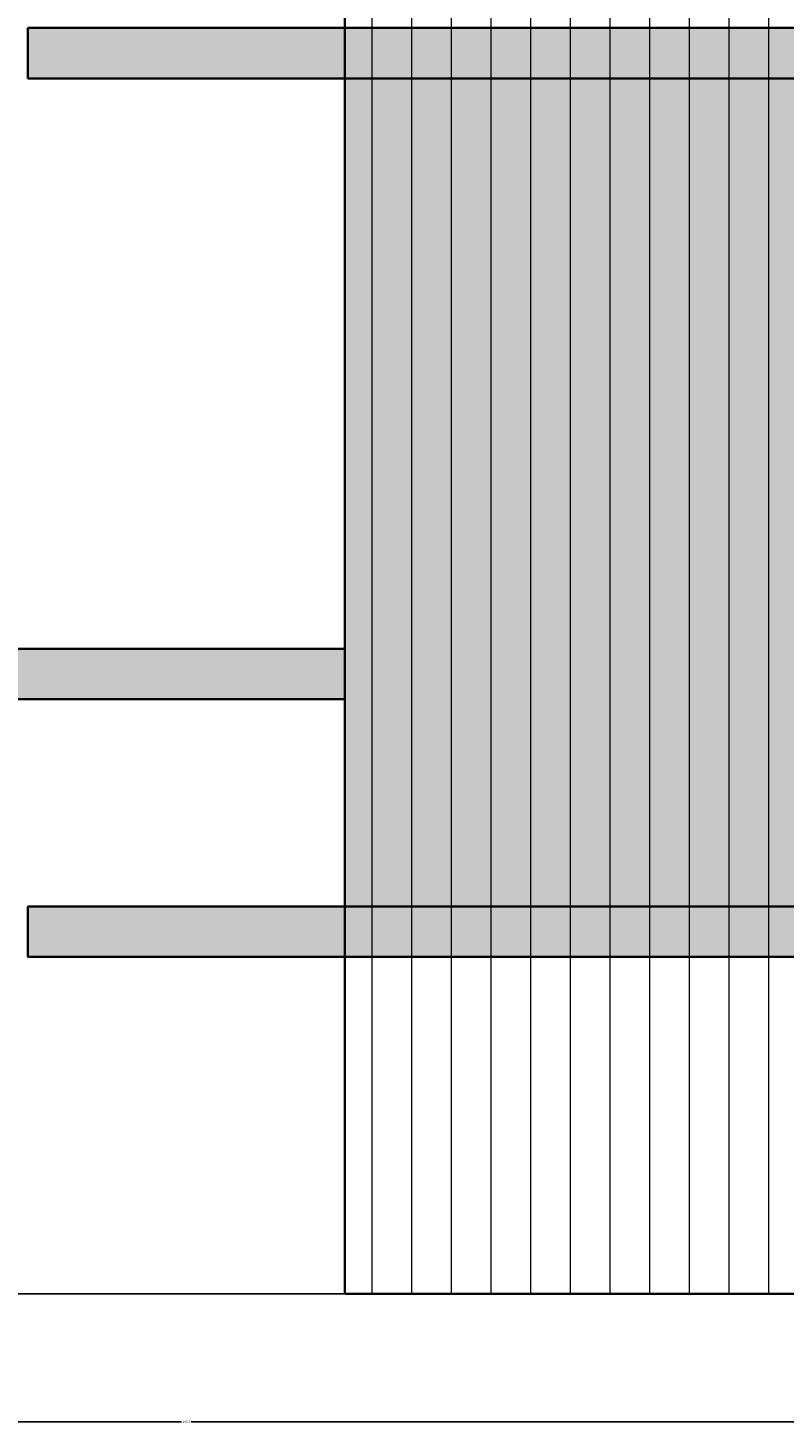
# Model space of a CAD drawing. Units: millimetres. Extents: x 446512 to 447461, y 70395 to 70610.
# Tile 33 of 39: x 447340 to 447401, y 70395 to 70507. Entities that reach past the tile are written whole.
import ezdxf

# ---------------------------------------------------------------- set-up
doc = ezdxf.new("R2010")
doc.units = ezdxf.units.MM
for name, color, linetype, lineweight in [('A-ANNO-DIMS', 2, 'Continuous', 18), ('A-FURN', 7, 'Continuous', 35), ('A-FURN-PATT', 38, 'Continuous', 13)]:
    doc.layers.add(name, color=color, linetype=linetype, lineweight=lineweight)
doc.styles.get("Standard").update_dxf_attribs({"font": 'arial.ttf'})
doc.dimstyles.get("Standard").update_dxf_attribs({"dimtxt": 0.18, "dimasz": 0.18, "dimexe": 0.18, "dimexo": 0.0625, "dimgap": 0.09, "dimtad": 0, "dimtih": 1, "dimtoh": 1, "dimdec": 4, "dimzin": 0, "dimdsep": 46, "dimtxsty": 'Standard', "dimcen": 0.09, "dimadec": 0, "dimazin": 0, "dimtfac": 1, "dimtdec": 4, "dimtofl": 0, "dimtmove": 0, "dimatfit": 3, "dimfxl": 1, "dimtolj": 1, "dimtzin": 0, "dimarcsym": 0})

# ---------------------------------------------------------------- blocks, each defined once
blk = doc.blocks.new('*D61')
at = {"layer": 'A-ANNO-DIMS', "color": 0, "lineweight": -2, "transparency": 16777216}
for p, q in [((447254.94, 70452.79), (447254.94, 70394.88)), ((447450.53, 70432.19), (447450.53, 70394.88)), ((447255.12, 70395.06), (447352.35, 70395.06)), ((447450.35, 70395.06), (447353.12, 70395.06))]:
    blk.add_line(p, q, dxfattribs=at)
at = {"layer": 'A-ANNO-DIMS', "color": 0, "transparency": 16777216}
for points in [[(447255.12, 70395.09), (447255.12, 70395.03), (447254.94, 70395.06)], [(447450.35, 70395.09), (447450.35, 70395.03), (447450.53, 70395.06)]]:
    blk.add_solid(points, dxfattribs=at)
at = {"layer": 'Defpoints', "color": 0, "transparency": 16777216}
for p in [(447254.94, 70452.85), (447450.53, 70432.25), (447450.53, 70395.06)]:
    blk.add_point(p, dxfattribs=at)
at = {"layer": 'A-ANNO-DIMS', "color": 0, "transparency": 16777216, "insert": (447352.74, 70395.06), "char_height": 0.18, "attachment_point": 5}
blk.add_mtext('\\A1;195.6', dxfattribs=at)
blk = doc.blocks.new('*D72')
at = {"layer": 'A-ANNO-DIMS', "color": 0, "lineweight": -2, "transparency": 16777216}
for p, q in [((447254.88, 70452.85), (447244.51, 70452.85)), ((447244.69, 70452.67), (447244.69, 70429.27)), ((447244.69, 70405.49), (447244.69, 70428.9)), ((447365.36, 70405.31), (447244.51, 70405.31))]:
    blk.add_line(p, q, dxfattribs=at)
at = {"layer": 'A-ANNO-DIMS', "color": 0, "transparency": 16777216}
for points in [[(447244.66, 70452.67), (447244.72, 70452.67), (447244.69, 70452.85)], [(447244.66, 70405.49), (447244.72, 70405.49), (447244.69, 70405.31)]]:
    blk.add_solid(points, dxfattribs=at)
at = {"layer": 'Defpoints', "color": 0, "transparency": 16777216}
for p in [(447244.69, 70452.85), (447254.94, 70452.85), (447365.43, 70405.31)]:
    blk.add_point(p, dxfattribs=at)
at = {"layer": 'A-ANNO-DIMS', "color": 0, "transparency": 16777216, "insert": (447244.69, 70429.08), "char_height": 0.18, "attachment_point": 5}
blk.add_mtext('\\A1;47.54', dxfattribs=at)

msp = doc.modelspace()

# ---------------------------------------------------------------- hatches: boundary and pattern name
at = {"layer": 'A-FURN-PATT'}
h = msp.add_hatch(dxfattribs=at)
h.set_pattern_fill('ANSI31', color=256, angle=45)
h.set_pattern_definition([(90, (127.5626, 0), (-3.175, 0), [])])
h.paths.add_polyline_path([(447426.0142, 70599.7147), (447365.4251, 70599.7147), (447365.4251, 70405.3145), (447426.0142, 70405.3145)])
h = msp.add_hatch(color=256, dxfattribs=at)
h.dxf.hatch_style = 1
h.paths.add_polyline_path([(447365.4251, 70506.5496), (447340.0494, 70506.5496), (447340.0494, 70502.5146), (447365.4251, 70502.5146)])
h.paths.add_polyline_path([(447450.5318, 70506.5496), (447426.0142, 70506.5496), (447426.0142, 70502.5146), (447450.5318, 70502.5146)])
h.paths.add_polyline_path([(447426.0142, 70506.5496), (447365.4251, 70506.5496), (447365.4251, 70502.5146), (447426.0142, 70502.5146)])
h = msp.add_hatch(color=256, dxfattribs=at)
h.dxf.hatch_style = 1
h.paths.add_polyline_path([(447426.0142, 70502.5146), (447365.4251, 70502.5146), (447365.4251, 70436.2876), (447426.0142, 70436.2876)])
h = msp.add_hatch(color=256, dxfattribs=at)
h.dxf.hatch_style = 1
h.paths.add_polyline_path([(447280.3184, 70456.89), (447254.9427, 70456.89), (447254.9427, 70452.855), (447280.3184, 70452.855)])
h.paths.add_polyline_path([(447365.4251, 70456.89), (447340.9075, 70456.89), (447340.9075, 70452.855), (447365.4251, 70452.855)])
h.paths.add_polyline_path([(447340.9075, 70456.89), (447280.3184, 70456.89), (447280.3184, 70452.855), (447340.9075, 70452.855)])
h = msp.add_hatch(color=256, dxfattribs=at)
h.dxf.hatch_style = 1
h.paths.add_polyline_path([(447365.4251, 70432.2526), (447365.4251, 70436.2876), (447340.0494, 70436.2876), (447340.0494, 70432.2526)])
h.paths.add_polyline_path([(447426.0142, 70436.2876), (447426.0142, 70432.2526), (447450.5318, 70432.2526), (447450.5318, 70436.2876)])
h = msp.add_hatch(color=256, dxfattribs=at)
h.dxf.hatch_style = 1
h.paths.add_polyline_path([(447426.0142, 70432.2526), (447426.0142, 70436.2876), (447365.4251, 70436.2876), (447365.4251, 70432.2526)])
h = msp.add_hatch(color=256, dxfattribs=at)
h.dxf.hatch_style = 1
h.paths.add_polyline_path([(447426.0142, 70432.2526), (447426.0142, 70436.2876), (447365.4251, 70436.2876), (447365.4251, 70432.2526)])
h = msp.add_hatch(color=256, dxfattribs=at)
h.dxf.hatch_style = 1
h.paths.add_polyline_path([(447426.0142, 70432.2526), (447426.0142, 70436.2876), (447365.4251, 70436.2876), (447365.4251, 70432.2526)])

# ---------------------------------------------------------------- linework, layer by layer
at = {"layer": 'A-FURN'}
for p, q in [((447365.4251, 70599.7147), (447365.4251, 70405.3145)), ((447365.4251, 70405.3145), (447426.0142, 70405.3145))]:
    msp.add_line(p, q, dxfattribs=at)
for points in [[(447340.0494, 70506.5496), (447450.5318, 70506.5496), (447450.5318, 70502.5146), (447340.0494, 70502.5146)], [(447254.9427, 70456.89), (447365.4251, 70456.89), (447365.4251, 70452.855), (447254.9427, 70452.855)], [(447340.0494, 70436.2876), (447450.5318, 70436.2876), (447450.5318, 70432.2526), (447340.0494, 70432.2526)]]:
    msp.add_lwpolyline(points, close=True, dxfattribs=at)

# ---------------------------------------------------------------- dimensions: what is measured, and where the dimension line sits
at = {"layer": 'A-ANNO-DIMS'}
dim = msp.add_linear_dim(base=(447244.6927, 70452.855), p1=(447365.4251, 70405.3145), p2=(447254.9427, 70452.855), angle=90, dimstyle='Standard', override={"dimdec": 2, "dimlfac": 1, "dimrnd": 0, "dimzin": 0, "dimdsep": 46, "dimlunit": 2}, dxfattribs=at)
dim.commit()
dim.dimension.update_dxf_attribs({"geometry": '*D72', "text_midpoint": (447244.6927, 70429.0848)})
dim = msp.add_linear_dim(base=(447450.5318, 70395.0645), p1=(447254.9427, 70452.855), p2=(447450.5318, 70432.2526), dimstyle='Standard', override={"dimdec": 1, "dimlfac": 1, "dimrnd": 0, "dimzin": 0, "dimdsep": 46, "dimlunit": 2}, dxfattribs=at)
dim.commit()
dim.dimension.update_dxf_attribs({"geometry": '*D61', "text_midpoint": (447352.7372, 70395.0645)})

doc.saveas('drawing.dxf')
